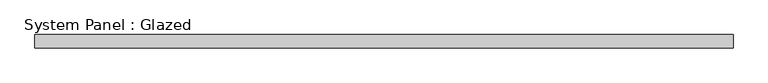
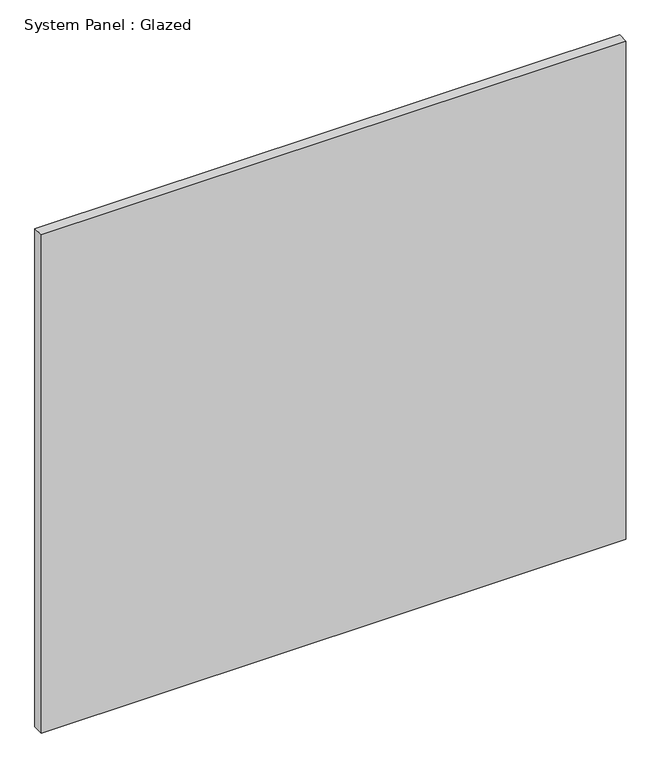
"""IFC4 building model written with IfcOpenShell, lengths in millimetres: plate geometry, System Panel : Glazed."""

from ifc_helpers import new_model, si_unit, origin, origin_with_axes, place, context, project, spatial, polyline, outline, extrude, source, transform, mapped, element, save


def system_panel_glazed_9f710733(model_context):
    return source(origin(), model_context, "Body", "SweptSolid", [
        extrude(outline(polyline([(676.7227528, 19.05), (-676.7227528, 19.05), (-676.7227528, 44.45), (676.7227528, 44.45), (676.7227528, 19.05)])), origin_with_axes(), (0.0, 0.0, 1.0), 1219.2),
    ])


if __name__ == "__main__":
    model = new_model("IFC4")
    model_context = context("Model", 3, world=origin())
    ifc_project = project(units=[si_unit("LENGTHUNIT", "METRE", prefix="MILLI")], contexts=[model_context])
    site = spatial("IfcSite", under=ifc_project)
    building = spatial("IfcBuilding", under=site)
    placement = place(None, origin())
    system_panel_glazed_shape = system_panel_glazed_9f710733(model_context)
    element("IfcPlate", 1, ObjectType="System Panel : Glazed", at=placement, inside=building, context=model_context, shape_type="MappedRepresentation", body=[
        mapped(system_panel_glazed_shape, transform((0.0, 0.0, 0.0), x_axis=(1.0, 0.0, 0.0), y_axis=(0.0, 1.0, 0.0), z_axis=(0.0, 0.0, 1.0))),
    ])
    save(model, "model.ifc")

# Revit data of these elements
# Type "System Panel : Glazed"
#   Construction Type Id = "GSP4R"
#   Analytic Construction = "1/8 in Pilkington single glazing"
#   Visual Light Transmittance = 0.9
#   Solar Heat Gain Coefficient = 0.86
#   Heat Transfer Coefficient (U) = 1.18115 BTU/(h·ft²·°F)
# Element 1 (IfcPlate, "System Panel : Glazed")
#   Materials on its faces: "Glass"
# Materials
#   "Glass": class "Glass", colour RGB 0 128 192, transparency 0.75, Description = "Soda Lime Glass", Cost = 0
